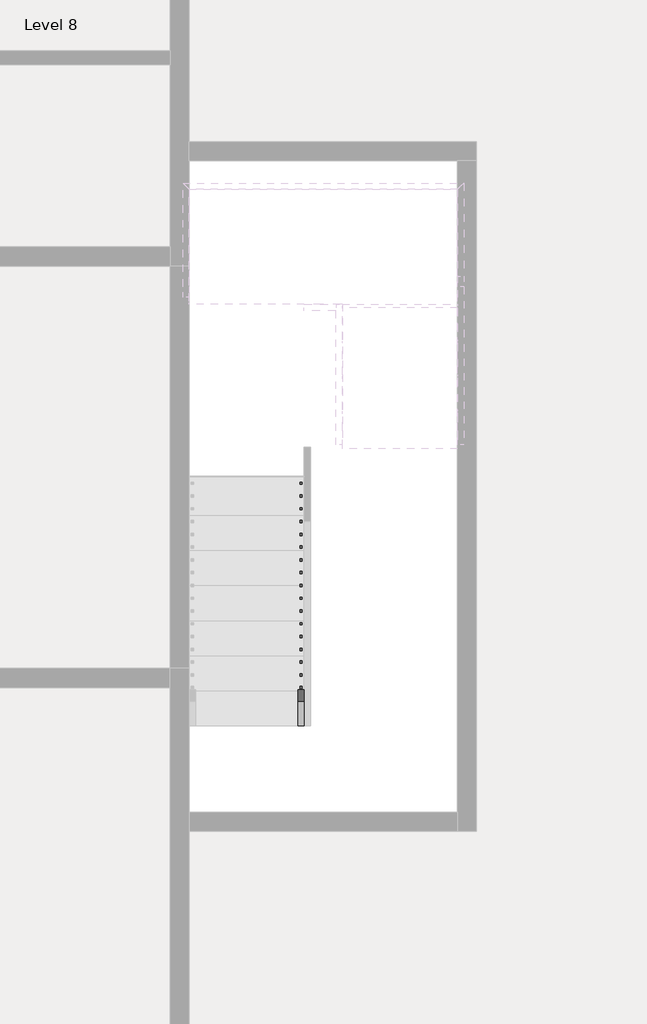
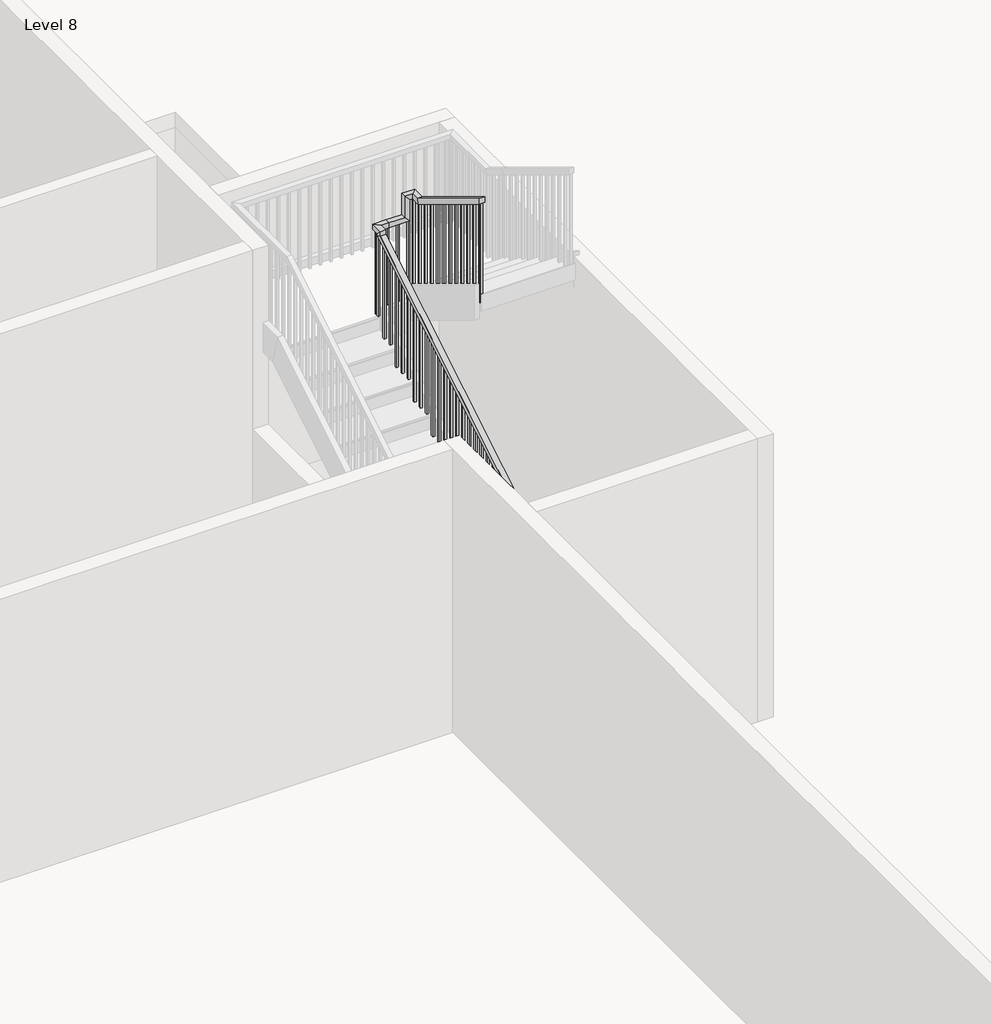
# One storey, part 7 of 8: 1 railing.
"""IFC4 building model written with IfcOpenShell, lengths in millimetres."""

from ifc_helpers import new_model, si_unit, frame, origin, place, context, project, spatial, polyline, outline, extrude, faceted_brep, element, save

model = new_model("IFC4")

# Units and contexts
model_context = context("Model", 3, world=origin())
ifc_project = project(units=[si_unit("LENGTHUNIT", "METRE", prefix="MILLI")], contexts=[model_context])

# Site, building, storey
site = spatial("IfcSite", under=ifc_project)
building = spatial("IfcBuilding", under=site)
storey = spatial("IfcBuildingStorey", under=building, Name="Level 8", Elevation=46570.6172466)

# Railing
placement = place(None, origin())
element("IfcRailing", 1, ObjectType="Handrail - Rectangular", at=placement, inside=storey, context=model_context, shape_type="SolidModel", body=[
    faceted_brep([(-2753.8415084, 19841.9216096, 47654.3505799), (-2753.8415084, 19841.9216096, 47594.9491197), (-2703.0415084, 19841.9216096, 47594.9491197), (-2703.0415084, 19841.9216096, 47654.3505799), (-2753.8415084, 23118.5216096, 49640.1687618), (-2753.8415084, 23169.3216096, 49611.5551803), (-2703.0415084, 23169.3216096, 49611.5551803), (-2703.0415084, 23118.5216096, 49640.1687618), (-2753.8415084, 23118.5216096, 49686.3505799), (-2753.8415084, 23169.3216096, 49635.5505799), (-2703.0415084, 23169.3216096, 49635.5505799), (-2703.0415084, 23118.5216096, 49686.3505799), (-2753.8415084, 23245.5216096, 49686.3505799), (-2753.8415084, 23245.5216096, 49635.5505799), (-2703.0415084, 23194.7216096, 49635.5505799), (-2703.0415084, 23194.7216096, 49686.3505799), (-2626.8415084, 23245.5216096, 49686.3505799), (-2626.8415084, 23245.5216096, 49635.5505799), (-2626.8415084, 23194.7216096, 49635.5505799), (-2626.8415084, 23194.7216096, 49686.3505799), (-2474.4415084, 23245.5216096, 49686.3505799), (-2423.6415084, 23245.5216096, 49635.5505799), (-2423.6415084, 23194.7216096, 49635.5505799), (-2474.4415084, 23194.7216096, 49686.3505799), (-2474.4415084, 23245.5216096, 49901.8657314), (-2423.6415084, 23245.5216096, 49851.0657314), (-2423.6415084, 23194.7216096, 49851.0657314), (-2474.4415084, 23194.7216096, 49901.8657314), (-2347.4415084, 23245.5216096, 49901.8657314), (-2347.4415084, 23245.5216096, 49851.0657314), (-2398.2415084, 23194.7216096, 49851.0657314), (-2398.2415084, 23194.7216096, 49901.8657314), (-2347.4415084, 23118.5216096, 49901.8657314), (-2347.4415084, 23104.3292002, 49851.0657314), (-2398.2415084, 23104.3292002, 49851.0657314), (-2398.2415084, 23118.5216096, 49901.8657314), (-2347.4415084, 22077.1216096, 50533.0172466), (-2398.2415084, 22077.1216096, 50533.0172466), (-2398.2415084, 22077.1216096, 50473.6157863), (-2347.4415084, 22077.1216096, 50473.6157863)], [[[0, 1, 2, 3]], [[1, 0, 4, 5]], [[2, 1, 5, 6]], [[3, 2, 6, 7]], [[0, 3, 7, 4]], [[5, 4, 8, 9]], [[6, 5, 9, 10]], [[7, 6, 10, 11]], [[4, 7, 11, 8]], [[9, 8, 12, 13]], [[10, 9, 13, 14]], [[11, 10, 14, 15]], [[8, 11, 15, 12]], [[13, 12, 16, 17]], [[14, 13, 17, 18]], [[15, 14, 18, 19]], [[12, 15, 19, 16]], [[17, 16, 20, 21]], [[18, 17, 21, 22]], [[19, 18, 22, 23]], [[16, 19, 23, 20]], [[21, 20, 24, 25]], [[22, 21, 25, 26]], [[23, 22, 26, 27]], [[20, 23, 27, 24]], [[25, 24, 28, 29]], [[26, 25, 29, 30]], [[27, 26, 30, 31]], [[24, 27, 31, 28]], [[29, 28, 32, 33]], [[30, 29, 33, 34]], [[31, 30, 34, 35]], [[28, 31, 35, 32]], [[36, 37, 38, 39]], [[33, 32, 36, 39]], [[34, 33, 39, 38]], [[35, 34, 38, 37]], [[32, 35, 37, 36]]]),
    extrude(outline(polyline([(22092.9966096, 50463.9945742), (22112.0466096, 50452.4491197), (22112.0466096, 49449.2839133), (22092.9966096, 49449.2839133), (22092.9966096, 50463.9945742)])), frame((-2382.3665084, 0.0, 0.0), z_axis=(1.0, 0.0, 0.0), x_axis=(0.0, 1.0, 0.0)), (0.0, 0.0, 1.0), 19.05),
    extrude(outline(polyline([(22194.5966096, 50402.4188166), (22213.6466096, 50390.8733621), (22213.6466096, 49449.2839133), (22194.5966096, 49449.2839133), (22194.5966096, 50402.4188166)])), frame((-2382.3665084, 0.0, 0.0), z_axis=(1.0, 0.0, 0.0), x_axis=(0.0, 1.0, 0.0)), (0.0, 0.0, 1.0), 19.05),
    extrude(outline(polyline([(22296.1966096, 50340.8430591), (22315.2466096, 50329.2976045), (22315.2466096, 49449.2839133), (22296.1966096, 49449.2839133), (22296.1966096, 50340.8430591)])), frame((-2382.3665084, 0.0, 0.0), z_axis=(1.0, 0.0, 0.0), x_axis=(0.0, 1.0, 0.0)), (0.0, 0.0, 1.0), 19.05),
    extrude(outline(polyline([(22397.7966096, 50279.2673015), (22416.8466096, 50267.721847), (22416.8466096, 49279.9505799), (22397.7966096, 49279.9505799), (22397.7966096, 50279.2673015)])), frame((-2382.3665084, 0.0, 0.0), z_axis=(1.0, 0.0, 0.0), x_axis=(0.0, 1.0, 0.0)), (0.0, 0.0, 1.0), 19.05),
    extrude(outline(polyline([(22499.3966096, 50217.6915439), (22518.4466096, 50206.1460894), (22518.4466096, 49279.9505799), (22499.3966096, 49279.9505799), (22499.3966096, 50217.6915439)])), frame((-2382.3665084, 0.0, 0.0), z_axis=(1.0, 0.0, 0.0), x_axis=(0.0, 1.0, 0.0)), (0.0, 0.0, 1.0), 19.05),
    extrude(outline(polyline([(22600.9966096, 50156.1157863), (22620.0466096, 50144.5703318), (22620.0466096, 49279.9505799), (22600.9966096, 49279.9505799), (22600.9966096, 50156.1157863)])), frame((-2382.3665084, 0.0, 0.0), z_axis=(1.0, 0.0, 0.0), x_axis=(0.0, 1.0, 0.0)), (0.0, 0.0, 1.0), 19.05),
    extrude(outline(polyline([(22702.5966096, 50094.5400288), (22721.6466096, 50082.9945742), (22721.6466096, 49110.6172466), (22702.5966096, 49110.6172466), (22702.5966096, 50094.5400288)])), frame((-2382.3665084, 0.0, 0.0), z_axis=(1.0, 0.0, 0.0), x_axis=(0.0, 1.0, 0.0)), (0.0, 0.0, 1.0), 19.05),
    extrude(outline(polyline([(22804.1966096, 50032.9642712), (22823.2466096, 50021.4188166), (22823.2466096, 49110.6172466), (22804.1966096, 49110.6172466), (22804.1966096, 50032.9642712)])), frame((-2382.3665084, 0.0, 0.0), z_axis=(1.0, 0.0, 0.0), x_axis=(0.0, 1.0, 0.0)), (0.0, 0.0, 1.0), 19.05),
    extrude(outline(polyline([(22905.7966096, 49971.3885136), (22924.8466096, 49959.8430591), (22924.8466096, 49110.6172466), (22905.7966096, 49110.6172466), (22905.7966096, 49971.3885136)])), frame((-2382.3665084, 0.0, 0.0), z_axis=(1.0, 0.0, 0.0), x_axis=(0.0, 1.0, 0.0)), (0.0, 0.0, 1.0), 19.05),
    extrude(outline(polyline([(23007.3966096, 49909.812756), (23026.4466096, 49898.2673015), (23026.4466096, 48941.2839133), (23007.3966096, 48941.2839133), (23007.3966096, 49909.812756)])), frame((-2382.3665084, 0.0, 0.0), z_axis=(1.0, 0.0, 0.0), x_axis=(0.0, 1.0, 0.0)), (0.0, 0.0, 1.0), 19.05),
    extrude(outline(polyline([(23108.9966096, 49848.2369985), (23128.0466096, 49836.6915439), (23128.0466096, 48941.2839133), (23108.9966096, 48941.2839133), (23108.9966096, 49848.2369985)])), frame((-2382.3665084, 0.0, 0.0), z_axis=(1.0, 0.0, 0.0), x_axis=(0.0, 1.0, 0.0)), (0.0, 0.0, 1.0), 19.05),
    extrude(outline(polyline([(-2433.1665084, 23210.5966096), (-2433.1665084, 23229.6466096), (-2414.1165084, 23229.6466096), (-2414.1165084, 23210.5966096), (-2433.1665084, 23210.5966096)])), frame((0.0, 0.0, 48771.9505799), z_axis=(0.0, 0.0, 1.0), x_axis=(1.0, 0.0, 0.0)), (0.0, 0.0, 1.0), 1079.1151515),
    extrude(outline(polyline([(-2534.7665084, 23210.5966096), (-2534.7665084, 23229.6466096), (-2515.7165084, 23229.6466096), (-2515.7165084, 23210.5966096), (-2534.7665084, 23210.5966096)])), frame((0.0, 0.0, 48771.9505799), z_axis=(0.0, 0.0, 1.0), x_axis=(1.0, 0.0, 0.0)), (0.0, 0.0, 1.0), 863.6),
    extrude(outline(polyline([(-2636.3665084, 23210.5966096), (-2636.3665084, 23229.6466096), (-2617.3165084, 23229.6466096), (-2617.3165084, 23210.5966096), (-2636.3665084, 23210.5966096)])), frame((0.0, 0.0, 48771.9505799), z_axis=(0.0, 0.0, 1.0), x_axis=(1.0, 0.0, 0.0)), (0.0, 0.0, 1.0), 863.6),
    extrude(outline(polyline([(-2718.9165084, 23185.1966096), (-2737.9665084, 23185.1966096), (-2737.9665084, 23204.2466096), (-2718.9165084, 23204.2466096), (-2718.9165084, 23185.1966096)])), frame((0.0, 0.0, 48771.9505799), z_axis=(0.0, 0.0, 1.0), x_axis=(1.0, 0.0, 0.0)), (0.0, 0.0, 1.0), 863.6),
    extrude(outline(polyline([(23083.5966096, 49559.6006348), (23102.6466096, 49571.1460894), (23102.6466096, 48602.6172466), (23083.5966096, 48602.6172466), (23083.5966096, 49559.6006348)])), frame((-2737.9665084, 0.0, 0.0), z_axis=(1.0, 0.0, 0.0), x_axis=(0.0, 1.0, 0.0)), (0.0, 0.0, 1.0), 19.05),
    extrude(outline(polyline([(22981.9966096, 49498.0248773), (23001.0466096, 49509.5703318), (23001.0466096, 48602.6172466), (22981.9966096, 48602.6172466), (22981.9966096, 49498.0248773)])), frame((-2737.9665084, 0.0, 0.0), z_axis=(1.0, 0.0, 0.0), x_axis=(0.0, 1.0, 0.0)), (0.0, 0.0, 1.0), 19.05),
    extrude(outline(polyline([(22880.3966096, 49436.4491197), (22899.4466096, 49447.9945742), (22899.4466096, 48433.2839133), (22880.3966096, 48433.2839133), (22880.3966096, 49436.4491197)])), frame((-2737.9665084, 0.0, 0.0), z_axis=(1.0, 0.0, 0.0), x_axis=(0.0, 1.0, 0.0)), (0.0, 0.0, 1.0), 19.05),
    extrude(outline(polyline([(22778.7966096, 49374.8733621), (22797.8466096, 49386.4188166), (22797.8466096, 48433.2839133), (22778.7966096, 48433.2839133), (22778.7966096, 49374.8733621)])), frame((-2737.9665084, 0.0, 0.0), z_axis=(1.0, 0.0, 0.0), x_axis=(0.0, 1.0, 0.0)), (0.0, 0.0, 1.0), 19.05),
    extrude(outline(polyline([(22677.1966096, 49313.2976045), (22696.2466096, 49324.8430591), (22696.2466096, 48433.2839133), (22677.1966096, 48433.2839133), (22677.1966096, 49313.2976045)])), frame((-2737.9665084, 0.0, 0.0), z_axis=(1.0, 0.0, 0.0), x_axis=(0.0, 1.0, 0.0)), (0.0, 0.0, 1.0), 19.05),
    extrude(outline(polyline([(22575.5966096, 49251.721847), (22594.6466096, 49263.2673015), (22594.6466096, 48263.9505799), (22575.5966096, 48263.9505799), (22575.5966096, 49251.721847)])), frame((-2737.9665084, 0.0, 0.0), z_axis=(1.0, 0.0, 0.0), x_axis=(0.0, 1.0, 0.0)), (0.0, 0.0, 1.0), 19.05),
    extrude(outline(polyline([(22473.9966096, 49190.1460894), (22493.0466096, 49201.6915439), (22493.0466096, 48263.9505799), (22473.9966096, 48263.9505799), (22473.9966096, 49190.1460894)])), frame((-2737.9665084, 0.0, 0.0), z_axis=(1.0, 0.0, 0.0), x_axis=(0.0, 1.0, 0.0)), (0.0, 0.0, 1.0), 19.05),
    extrude(outline(polyline([(22372.3966096, 49128.5703318), (22391.4466096, 49140.1157863), (22391.4466096, 48263.9505799), (22372.3966096, 48263.9505799), (22372.3966096, 49128.5703318)])), frame((-2737.9665084, 0.0, 0.0), z_axis=(1.0, 0.0, 0.0), x_axis=(0.0, 1.0, 0.0)), (0.0, 0.0, 1.0), 19.05),
    extrude(outline(polyline([(22270.7966096, 49066.9945742), (22289.8466096, 49078.5400288), (22289.8466096, 48094.6172466), (22270.7966096, 48094.6172466), (22270.7966096, 49066.9945742)])), frame((-2737.9665084, 0.0, 0.0), z_axis=(1.0, 0.0, 0.0), x_axis=(0.0, 1.0, 0.0)), (0.0, 0.0, 1.0), 19.05),
    extrude(outline(polyline([(22169.1966096, 49005.4188166), (22188.2466096, 49016.9642712), (22188.2466096, 48094.6172466), (22169.1966096, 48094.6172466), (22169.1966096, 49005.4188166)])), frame((-2737.9665084, 0.0, 0.0), z_axis=(1.0, 0.0, 0.0), x_axis=(0.0, 1.0, 0.0)), (0.0, 0.0, 1.0), 19.05),
    extrude(outline(polyline([(22067.5966096, 48943.8430591), (22086.6466096, 48955.3885136), (22086.6466096, 48094.6172466), (22067.5966096, 48094.6172466), (22067.5966096, 48943.8430591)])), frame((-2737.9665084, 0.0, 0.0), z_axis=(1.0, 0.0, 0.0), x_axis=(0.0, 1.0, 0.0)), (0.0, 0.0, 1.0), 19.05),
    extrude(outline(polyline([(21965.9966096, 48882.2673015), (21985.0466096, 48893.812756), (21985.0466096, 47925.2839133), (21965.9966096, 47925.2839133), (21965.9966096, 48882.2673015)])), frame((-2737.9665084, 0.0, 0.0), z_axis=(1.0, 0.0, 0.0), x_axis=(0.0, 1.0, 0.0)), (0.0, 0.0, 1.0), 19.05),
    extrude(outline(polyline([(21864.3966096, 48820.6915439), (21883.4466096, 48832.2369985), (21883.4466096, 47925.2839133), (21864.3966096, 47925.2839133), (21864.3966096, 48820.6915439)])), frame((-2737.9665084, 0.0, 0.0), z_axis=(1.0, 0.0, 0.0), x_axis=(0.0, 1.0, 0.0)), (0.0, 0.0, 1.0), 19.05),
    extrude(outline(polyline([(21762.7966096, 48759.1157863), (21781.8466096, 48770.6612409), (21781.8466096, 47755.9505799), (21762.7966096, 47755.9505799), (21762.7966096, 48759.1157863)])), frame((-2737.9665084, 0.0, 0.0), z_axis=(1.0, 0.0, 0.0), x_axis=(0.0, 1.0, 0.0)), (0.0, 0.0, 1.0), 19.05),
    extrude(outline(polyline([(21661.1966096, 48697.5400288), (21680.2466096, 48709.0854833), (21680.2466096, 47755.9505799), (21661.1966096, 47755.9505799), (21661.1966096, 48697.5400288)])), frame((-2737.9665084, 0.0, 0.0), z_axis=(1.0, 0.0, 0.0), x_axis=(0.0, 1.0, 0.0)), (0.0, 0.0, 1.0), 19.05),
    extrude(outline(polyline([(21559.5966096, 48635.9642712), (21578.6466096, 48647.5097257), (21578.6466096, 47755.9505799), (21559.5966096, 47755.9505799), (21559.5966096, 48635.9642712)])), frame((-2737.9665084, 0.0, 0.0), z_axis=(1.0, 0.0, 0.0), x_axis=(0.0, 1.0, 0.0)), (0.0, 0.0, 1.0), 19.05),
    extrude(outline(polyline([(21457.9966096, 48574.3885136), (21477.0466096, 48585.9339682), (21477.0466096, 47586.6172466), (21457.9966096, 47586.6172466), (21457.9966096, 48574.3885136)])), frame((-2737.9665084, 0.0, 0.0), z_axis=(1.0, 0.0, 0.0), x_axis=(0.0, 1.0, 0.0)), (0.0, 0.0, 1.0), 19.05),
    extrude(outline(polyline([(21356.3966096, 48512.812756), (21375.4466096, 48524.3582106), (21375.4466096, 47586.6172466), (21356.3966096, 47586.6172466), (21356.3966096, 48512.812756)])), frame((-2737.9665084, 0.0, 0.0), z_axis=(1.0, 0.0, 0.0), x_axis=(0.0, 1.0, 0.0)), (0.0, 0.0, 1.0), 19.05),
    extrude(outline(polyline([(21254.7966096, 48451.2369985), (21273.8466096, 48462.782453), (21273.8466096, 47586.6172466), (21254.7966096, 47586.6172466), (21254.7966096, 48451.2369985)])), frame((-2737.9665084, 0.0, 0.0), z_axis=(1.0, 0.0, 0.0), x_axis=(0.0, 1.0, 0.0)), (0.0, 0.0, 1.0), 19.05),
    extrude(outline(polyline([(21153.1966096, 48389.6612409), (21172.2466096, 48401.2066954), (21172.2466096, 47417.2839133), (21153.1966096, 47417.2839133), (21153.1966096, 48389.6612409)])), frame((-2737.9665084, 0.0, 0.0), z_axis=(1.0, 0.0, 0.0), x_axis=(0.0, 1.0, 0.0)), (0.0, 0.0, 1.0), 19.05),
    extrude(outline(polyline([(21051.5966096, 48328.0854833), (21070.6466096, 48339.6309379), (21070.6466096, 47417.2839133), (21051.5966096, 47417.2839133), (21051.5966096, 48328.0854833)])), frame((-2737.9665084, 0.0, 0.0), z_axis=(1.0, 0.0, 0.0), x_axis=(0.0, 1.0, 0.0)), (0.0, 0.0, 1.0), 19.05),
    extrude(outline(polyline([(20949.9966096, 48266.5097257), (20969.0466096, 48278.0551803), (20969.0466096, 47417.2839133), (20949.9966096, 47417.2839133), (20949.9966096, 48266.5097257)])), frame((-2737.9665084, 0.0, 0.0), z_axis=(1.0, 0.0, 0.0), x_axis=(0.0, 1.0, 0.0)), (0.0, 0.0, 1.0), 19.05),
    extrude(outline(polyline([(20848.3966096, 48204.9339682), (20867.4466096, 48216.4794227), (20867.4466096, 47247.9505799), (20848.3966096, 47247.9505799), (20848.3966096, 48204.9339682)])), frame((-2737.9665084, 0.0, 0.0), z_axis=(1.0, 0.0, 0.0), x_axis=(0.0, 1.0, 0.0)), (0.0, 0.0, 1.0), 19.05),
    extrude(outline(polyline([(20746.7966096, 48143.3582106), (20765.8466096, 48154.9036651), (20765.8466096, 47247.9505799), (20746.7966096, 47247.9505799), (20746.7966096, 48143.3582106)])), frame((-2737.9665084, 0.0, 0.0), z_axis=(1.0, 0.0, 0.0), x_axis=(0.0, 1.0, 0.0)), (0.0, 0.0, 1.0), 19.05),
    extrude(outline(polyline([(20645.1966096, 48081.782453), (20664.2466096, 48093.3279076), (20664.2466096, 47078.6172466), (20645.1966096, 47078.6172466), (20645.1966096, 48081.782453)])), frame((-2737.9665084, 0.0, 0.0), z_axis=(1.0, 0.0, 0.0), x_axis=(0.0, 1.0, 0.0)), (0.0, 0.0, 1.0), 19.05),
    extrude(outline(polyline([(20543.5966096, 48020.2066954), (20562.6466096, 48031.75215), (20562.6466096, 47078.6172466), (20543.5966096, 47078.6172466), (20543.5966096, 48020.2066954)])), frame((-2737.9665084, 0.0, 0.0), z_axis=(1.0, 0.0, 0.0), x_axis=(0.0, 1.0, 0.0)), (0.0, 0.0, 1.0), 19.05),
    extrude(outline(polyline([(20441.9966096, 47958.6309379), (20461.0466096, 47970.1763924), (20461.0466096, 47078.6172466), (20441.9966096, 47078.6172466), (20441.9966096, 47958.6309379)])), frame((-2737.9665084, 0.0, 0.0), z_axis=(1.0, 0.0, 0.0), x_axis=(0.0, 1.0, 0.0)), (0.0, 0.0, 1.0), 19.05),
    extrude(outline(polyline([(20340.3966096, 47897.0551803), (20359.4466096, 47908.6006348), (20359.4466096, 46909.2839133), (20340.3966096, 46909.2839133), (20340.3966096, 47897.0551803)])), frame((-2737.9665084, 0.0, 0.0), z_axis=(1.0, 0.0, 0.0), x_axis=(0.0, 1.0, 0.0)), (0.0, 0.0, 1.0), 19.05),
    extrude(outline(polyline([(20238.7966096, 47835.4794227), (20257.8466096, 47847.0248773), (20257.8466096, 46909.2839133), (20238.7966096, 46909.2839133), (20238.7966096, 47835.4794227)])), frame((-2737.9665084, 0.0, 0.0), z_axis=(1.0, 0.0, 0.0), x_axis=(0.0, 1.0, 0.0)), (0.0, 0.0, 1.0), 19.05),
    extrude(outline(polyline([(20137.1966096, 47773.9036651), (20156.2466096, 47785.4491197), (20156.2466096, 46909.2839133), (20137.1966096, 46909.2839133), (20137.1966096, 47773.9036651)])), frame((-2737.9665084, 0.0, 0.0), z_axis=(1.0, 0.0, 0.0), x_axis=(0.0, 1.0, 0.0)), (0.0, 0.0, 1.0), 19.05),
    extrude(outline(polyline([(20035.5966096, 47712.3279076), (20054.6466096, 47723.8733621), (20054.6466096, 46739.9505799), (20035.5966096, 46739.9505799), (20035.5966096, 47712.3279076)])), frame((-2737.9665084, 0.0, 0.0), z_axis=(1.0, 0.0, 0.0), x_axis=(0.0, 1.0, 0.0)), (0.0, 0.0, 1.0), 19.05),
    extrude(outline(polyline([(19933.9966096, 47650.75215), (19953.0466096, 47662.2976045), (19953.0466096, 46739.9505799), (19933.9966096, 46739.9505799), (19933.9966096, 47650.75215)])), frame((-2737.9665084, 0.0, 0.0), z_axis=(1.0, 0.0, 0.0), x_axis=(0.0, 1.0, 0.0)), (0.0, 0.0, 1.0), 19.05),
    extrude(outline(polyline([(-2382.3665084, 23210.5966096), (-2382.3665084, 23229.6466096), (-2363.3165084, 23229.6466096), (-2363.3165084, 23210.5966096), (-2382.3665084, 23210.5966096)])), frame((0.0, 0.0, 48771.9505799), z_axis=(0.0, 0.0, 1.0), x_axis=(1.0, 0.0, 0.0)), (0.0, 0.0, 1.0), 1079.1151515),
    extrude(outline(polyline([(-2718.9165084, 23210.5966096), (-2737.9665084, 23210.5966096), (-2737.9665084, 23229.6466096), (-2718.9165084, 23229.6466096), (-2718.9165084, 23210.5966096)])), frame((0.0, 0.0, 48771.9505799), z_axis=(0.0, 0.0, 1.0), x_axis=(1.0, 0.0, 0.0)), (0.0, 0.0, 1.0), 863.6),
    extrude(outline(polyline([(22077.1216096, 50473.6157863), (22096.1716096, 50462.0703318), (22096.1716096, 49449.2839133), (22077.1216096, 49449.2839133), (22077.1216096, 50473.6157863)])), frame((-2382.3665084, 0.0, 0.0), z_axis=(1.0, 0.0, 0.0), x_axis=(0.0, 1.0, 0.0)), (0.0, 0.0, 1.0), 19.05),
    extrude(outline(polyline([(19841.9216096, 47594.9491197), (19860.9716096, 47606.4945742), (19860.9716096, 46739.9505799), (19841.9216096, 46739.9505799), (19841.9216096, 47594.9491197)])), frame((-2737.9665084, 0.0, 0.0), z_axis=(1.0, 0.0, 0.0), x_axis=(0.0, 1.0, 0.0)), (0.0, 0.0, 1.0), 19.05),
])

save(model, "model.ifc")

# Revit data of these elements
# Type "Handrail - Rectangular"
#   Assembly Code = "C2010400"
#   built-in parameter 1008612 = 0.0416667 (stored number, unit not read)
#   built-in parameter 1008611 = 0.0416667 (stored number, unit not read)
#   built-in parameter 1008609 = 0.333333 (stored number, unit not read)
#   built-in parameter 1008604 = 0.166667 (stored number, unit not read)
#   built-in parameter 1008603 = 0.166667 (stored number, unit not read)
#   Railing Height = 3' - 0"
#   built-in parameter 1008630 = 2
#   built-in parameter 1008610 = 2
#   built-in parameter 1008618 = Baluster - Square : 3/4"
# Element 1 (IfcRailing, "Handrail - Rectangular")
#   Phase Created = New Construction
